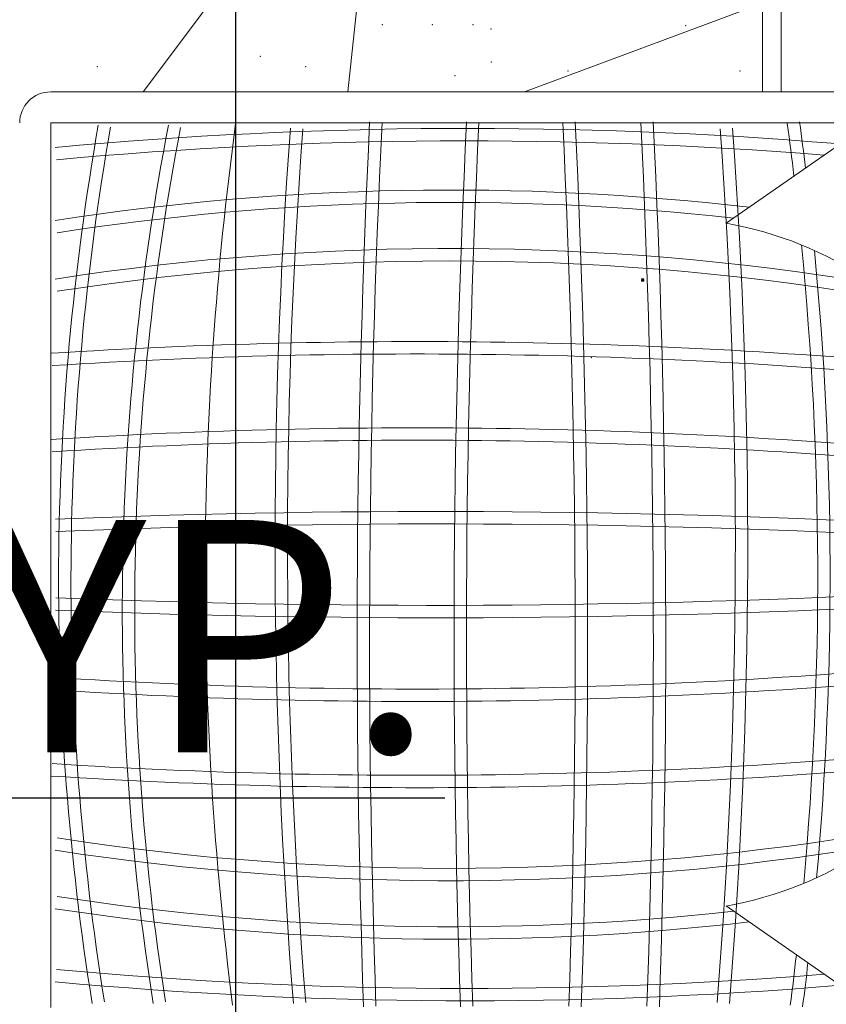
# Model space of a CAD drawing. Units: inches. Extents: x 1763 to 2368, y 1500 to 2097.
# Tile 19 of 24: x 2109 to 2152, y 1882 to 1935. Entities that reach past the tile are written whole.
import ezdxf

# ---------------------------------------------------------------- set-up
doc = ezdxf.new("R2010")
doc.units = ezdxf.units.IN
for name, color, linetype, lineweight in [('A-ANNO-DIMS', 2, 'Continuous', 18), ('A-FURN', 8, 'Continuous', 18), ('A-WALL-PATT', 7, 'Continuous', 13)]:
    doc.layers.add(name, color=color, linetype=linetype, lineweight=lineweight)
doc.styles.get("Standard").update_dxf_attribs({"font": 'arial.ttf'})
doc.dimstyles.new('ISO-25', dxfattribs={"dimtxt": 12.5, "dimasz": 2.5, "dimexe": 1.25, "dimexo": 0.625, "dimtad": 1, "dimdec": 0, "dimlunit": 4, "dimtxsty": 'Standard', "dimblk": 'ARCHTICK', "dimcen": 2.5, "dimclrd": 3, "dimclrt": 4, "dimadec": 0, "dimazin": 0, "dimtfac": 1, "dimtdec": 0, "dimtmove": 0, "dimatfit": 3, "dimfxl": 1, "dimarcsym": 0})

# ---------------------------------------------------------------- blocks, each defined once
blk = doc.blocks.new('A$C4CB008C5')
for p, q in [((0, 3), (0.6, 3)), ((0, 2.6), (0, 3)), ((0.6, 2.6), (0, 2.6)), ((0.1, 2.8), (0.5, 2.8)), ((0.1, 1.5), (0.6, 1.5)), ((0.1, 1.5), (0.1, 1.5)), ((0.1, 1.5), (0.1, 1.5)), ((0.1, 1.5), (0.1, 1.5)), ((0.1, 1.4), (0.1, 1.5)), ((0.1, 1.4), (0.1, 1.5)), ((0.1, 1.5), (0.1, 1.5)), ((0.1, 1.5), (0.1, 1.5)), ((0.1, 1.5), (0.1, 1.5)), ((0.1, 1.5), (0.1, 1.5)), ((0.1, 0), (0.1, 1.5)), ((0.1, 1.4), (0.1, 1.4)), ((0.1, 1.4), (0.1, 1.4)), ((0.1, 1.4), (0.1, 1.4)), ((0.1, 1.3), (0.1, 1.4)), ((0.1, 1.3), (0.1, 1.4)), ((0.1, 1.3), (0.1, 1.4)), ((0.1, 1.3), (0.1, 1.3)), ((0.1, 1.3), (0.1, 1.4)), ((0.1, 1.4), (0.1, 1.4)), ((0.1, 1.4), (0.1, 1.4)), ((0.1, 1.4), (0.1, 1.4)), ((0.1, 1.4), (0.1, 1.4)), ((0.1, 1.3), (0.1, 1.3)), ((0.1, 1.3), (0.1, 1.3)), ((0.1, 1.3), (0.1, 1.3)), ((0.1, 1.2), (0.1, 1.3)), ((0.1, 1.2), (0.1, 1.3)), ((0.1, 1.2), (0.1, 1.3)), ((0.1, 1.2), (0.1, 1.3)), ((0.1, 1.2), (0.1, 1.3)), ((0.1, 1.3), (0.1, 1.3)), ((0.1, 1.3), (0.1, 1.3)), ((0.1, 1.3), (0.1, 1.3)), ((0.1, 1.2), (0.1, 1.2)), ((0.1, 1.2), (0.1, 1.2)), ((0.1, 1.2), (0.1, 1.2)), ((0.1, 1.1), (0.1, 1.2)), ((0.1, 1.1), (0.1, 1.2)), ((0.1, 1.1), (0.1, 1.2)), ((0.1, 1.2), (0.1, 1.2)), ((0.1, 1.2), (0.1, 1.2)), ((0.1, 1.2), (0.1, 1.2)), ((0.1, 1.2), (0.1, 1.2)), ((0.1, 1.1), (0.1, 1.1)), ((0.1, 1.1), (0.1, 1.1)), ((0.1, 1.1), (0.1, 1.1)), ((0.1, 1), (0.1, 1.1)), ((0.1, 1), (0.1, 1.1)), ((0.1, 1), (0.1, 1)), ((0.1, 1), (0.1, 1.1)), ((0.1, 1.1), (0.1, 1.1)), ((0.1, 1.1), (0.1, 1.1)), ((0.1, 1.1), (0.1, 1.1)), ((0.1, 1), (0.1, 1)), ((0.1, 1), (0.1, 1)), ((0.1, 1), (0.1, 1)), ((0.1, 0.9), (0.1, 1)), ((0.1, 0.9), (0.1, 1)), ((0.1, 0.9), (0.1, 1)), ((0.1, 0.9), (0.1, 1)), ((0.1, 0.9), (0.1, 1)), ((0.1, 0.9), (0.1, 1)), ((0.1, 1), (0.1, 1)), ((0.1, 1), (0.1, 1)), ((0.1, 1), (0.1, 1)), ((0.1, 0.9), (0.1, 0.9)), ((0.1, 0.9), (0.1, 0.9)), ((0.1, 0.9), (0.1, 0.9)), ((0.1, 0.8), (0.1, 0.9)), ((0.1, 0.8), (0.1, 0.9)), ((0.1, 0.8), (0.1, 0.9)), ((0.1, 0.8), (0.1, 0.9)), ((0.1, 0.9), (0.1, 0.9)), ((0.1, 0.9), (0.1, 0.9)), ((0.1, 0.9), (0.1, 0.9)), ((0.1, 0.9), (0.1, 0.9)), ((0.1, 0.8), (0.1, 0.8)), ((0.1, 0.8), (0.1, 0.8)), ((0.1, 0.7), (0.1, 0.8)), ((0.1, 0.7), (0.1, 0.8)), ((0.1, 0.7), (0.1, 0.8)), ((0.1, 0.8), (0.1, 0.8)), ((0.1, 0.8), (0.1, 0.8)), ((0.1, 0.8), (0.1, 0.8)), ((0.1, 0.8), (0.1, 0.8)), ((0.1, 0.7), (0.1, 0.7)), ((0.1, 0.7), (0.1, 0.7)), ((0.1, 0.7), (0.1, 0.7)), ((0.1, 0.6), (0.1, 0.7)), ((0.1, 0.6), (0.1, 0.7)), ((0.1, 0.6), (0.1, 0.7)), ((0.1, 0.6), (0.1, 0.7)), ((0.1, 0.6), (0.1, 0.7)), ((0.1, 0.7), (0.1, 0.7)), ((0.1, 0.7), (0.1, 0.7)), ((0.1, 0.7), (0.1, 0.7)), ((0.1, 0.6), (0.1, 0.6)), ((0.1, 0.6), (0.1, 0.6)), ((0.1, 0.6), (0.1, 0.6)), ((0.1, 0.5), (0.1, 0.6)), ((0.1, 0.5), (0.1, 0.6)), ((0.1, 0.5), (0.1, 0.6)), ((0.1, 0.5), (0.1, 0.6)), ((0.1, 0.5), (0.1, 0.6)), ((0.1, 0.6), (0.1, 0.6)), ((0.1, 0.6), (0.1, 0.6)), ((0.1, 0.6), (0.1, 0.6)), ((0.1, 0.6), (0.1, 0.6)), ((0.1, 0.5), (0.1, 0.5)), ((0.1, 0.5), (0.1, 0.5)), ((0.1, 0.4), (0.1, 0.5)), ((0.1, 0.4), (0.1, 0.5)), ((0.1, 0.5), (0.1, 0.5)), ((0.1, 0.5), (0.1, 0.5)), ((0.1, 0.5), (0.1, 0.5)), ((0.1, 0.5), (0.1, 0.5)), ((0.1, 0.4), (0.1, 0.4)), ((0.1, 0.4), (0.1, 0.4)), ((0.1, 0.4), (0.1, 0.4)), ((0.1, 0.4), (0.1, 0.4)), ((0.1, 0.3), (0.1, 0.4)), ((0.1, 0.3), (0.1, 0.4)), ((0.1, 0.3), (0.1, 0.4)), ((0.1, 0.3), (0.1, 0.4)), ((0.1, 0.4), (0.1, 0.4)), ((0.1, 0.4), (0.1, 0.4)), ((0.1, 0.4), (0.1, 0.4)), ((0.1, 0.3), (0.1, 0.3)), ((0.1, 0.3), (0.1, 0.3)), ((0.1, 0.3), (0.1, 0.3)), ((0.1, 0.2), (0.1, 0.3)), ((0.1, 0.2), (0.1, 0.3)), ((0.1, 0.2), (0.1, 0.3)), ((0.1, 0.2), (0.1, 0.3)), ((0.1, 0.2), (0.1, 0.3)), ((0.1, 0.2), (0.1, 0.3)), ((0.1, 0.3), (0.1, 0.3)), ((0.1, 0.3), (0.1, 0.3)), ((0.1, 0.3), (0.1, 0.3)), ((0.1, 0.3), (0.1, 0.3)), ((0.1, 0.2), (0.1, 0.2)), ((0.1, 0.2), (0.1, 0.2)), ((0.1, 0.1), (0.1, 0.2)), ((0.1, 0.1), (0.1, 0.2)), ((0.1, 0.1), (0.1, 0.2)), ((0.1, 0.2), (0.1, 0.2)), ((0.1, 0.2), (0.1, 0.2)), ((0.1, 0.2), (0.1, 0.2)), ((0.1, 0.2), (0.1, 0.2)), ((0.1, 0.1), (0.1, 0.1)), ((0.1, 0.1), (0.1, 0.1)), ((0.1, 0.1), (0.1, 0.1)), ((0.1, 0), (0.1, 0.1)), ((0.1, 0), (0.1, 0.1)), ((0.1, 0.1), (0.1, 0.1)), ((0.1, 0), (0.1, 0.1)), ((0.1, 0.1), (0.1, 0.1)), ((0.1, 0.1), (0.1, 0.1)), ((0.1, 0.1), (0.1, 0.1)), ((0.1, 0), (0.1, 0)), ((0.1, 0), (0.1, 0)), ((0.1, 0), (0.1, 0)), ((0.1, 0), (0.1, 0)), ((0.1, 0), (0.1, 0)), ((0.1, 0), (0.1, 0)), ((0.1, 0), (0.1, 0)), ((0.3, 2.6), (0.3, 3)), ((0.3, 1.1), (0.5, 1.3)), ((0.7, 0.9), (0.3, 1.3)), ((0.3, 0.1), (0.3, 1.3)), ((0.3, 1.3), (0.6, 1.3)), ((0.3, 0.8), (0.6, 1.2)), ((0.6, 0.7), (0.3, 1)), ((0.3, 0.5), (0.6, 0.9)), ((0.9, 0.1), (0.3, 0.7)), ((0.3, 0.3), (0.6, 0.6)), ((0.6, 0.1), (0.3, 0.5)), ((0.3, 0.1), (0.3, 0.2)), ((3, 0.1), (0.3, 0.1)), ((0.6, 1.2), (0.5, 1.3)), ((0.5, 0.1), (0.8, 0.5)), ((0.6, 3), (2.6, 3)), ((0.6, 1.1), (0.6, 3)), ((0.6, 3), (2.6, 3)), ((0.6, 3), (0.6, 2.6)), ((0.6, 2.1), (1.9, 2.7)), ((0.6, 0.9), (0.6, 0.5)), ((2.5, 1), (0.7, 1)), ((0.7, 0.9), (0.8, 1)), ((0.7, 0.9), (2.6, 0.9)), ((0.7, 0.5), (2.6, 0.5)), ((0.7, 0.1), (1.1, 0.5)), ((0.8, 2.9), (1.6, 2.9)), ((0.8, 2.9), (2.5, 2.9)), ((0.8, 2.5), (0.8, 2.9)), ((0.8, 2.5), (0.8, 2.9)), ((0.8, 2.9), (0.8, 2.9)), ((1.6, 2.5), (0.8, 2.5)), ((0.8, 2.5), (0.8, 2.5)), ((1.5, 2.5), (0.8, 2.5)), ((1.2, 0.1), (0.8, 0.5)), ((0.9, 1.9), (1.9, 2.7)), ((0.9, 1.9), (0.9, 1.9)), ((1, 0.9), (0.9, 1)), ((1, 0.9), (1.1, 1)), ((1, 0.1), (1.4, 0.5)), ((1.2, 0.9), (1.1, 1)), ((1.4, 0.1), (1.1, 0.5)), ((1.2, 0.9), (1.3, 1)), ((1.3, 0.1), (1.6, 0.5)), ((1.5, 0.9), (1.4, 1)), ((1.7, 0.1), (1.4, 0.5)), ((1.5, 0.9), (1.6, 1)), ((1.6, 2.9), (1.6, 2.6)), ((1.6, 2.9), (1.7, 2.9)), ((1.6, 0.1), (1.9, 0.5)), ((1.7, 2.9), (1.7, 2.6)), ((1.7, 2.9), (1.7, 2.6)), ((1.7, 2.9), (2.5, 2.9)), ((1.7, 2.9), (1.7, 2.9)), ((1.8, 0.9), (1.7, 1)), ((2, 0.1), (1.7, 0.5)), ((1.8, 0.9), (1.9, 1)), ((1.9, 2.7), (2.6, 2.5)), ((1.9, 2.7), (2.5, 2.4)), ((1.9, 0.1), (2.2, 0.5)), ((2.1, 0.9), (2, 1)), ((2.3, 0.1), (2, 0.5)), ((2.1, 0.9), (2.2, 1)), ((2.2, 0.1), (2.5, 0.5)), ((2.4, 0.9), (2.3, 1)), ((2.6, 0.1), (2.3, 0.5)), ((2.4, 0.9), (2.5, 1)), ((2.4, 0.1), (3, 0.7)), ((2.5, 2.9), (2.5, 2.5)), ((2.5, 2.9), (2.5, 2.6)), ((2.5, 2.9), (2.5, 2.9)), ((2.9, 0.1), (2.5, 0.5)), ((2.6, 3), (2.6, 1.1)), ((2.6, 1.5), (3.2, 1.5)), ((2.6, 1.2), (2.8, 1.3)), ((2.6, 0.9), (3, 1.3)), ((2.6, 1.3), (3, 1.3)), ((3, 0.9), (2.6, 1.2)), ((2.6, 0.6), (3, 1)), ((3, 0.6), (2.6, 1)), ((2.6, 0.9), (2.6, 0.5)), ((3, 0.3), (2.6, 0.7)), ((3.3, 3), (2.7, 3)), ((2.7, 3), (2.7, 2.6)), ((2.7, 2.6), (3.3, 2.6)), ((2.7, 0.1), (3, 0.4)), ((3.2, 2.8), (2.8, 2.8)), ((3, 1.2), (2.8, 1.3)), ((3, 2.6), (3, 3)), ((3, 1.3), (3, 0.1)), ((3.2, 1.5), (3.1, 1.5)), ((3.1, 1.5), (3.1, 1.5)), ((3.1, 1.5), (3.2, 1.5)), ((3.1, 1.5), (3.2, 1.5)), ((3.1, 1.5), (3.1, 0)), ((3.2, 1.3), (3.1, 1.4)), ((3.2, 1.3), (3.1, 1.4)), ((3.2, 1.3), (3.1, 1.4)), ((3.2, 1.4), (3.1, 1.4)), ((3.2, 1.4), (3.1, 1.4)), ((3.1, 1.4), (3.1, 1.4)), ((3.1, 1.4), (3.2, 1.4)), ((3.1, 1.4), (3.2, 1.4)), ((3.1, 1.4), (3.2, 1.4)), ((3.1, 1.3), (3.2, 1.4)), ((3.1, 1.3), (3.2, 1.3)), ((3.2, 1.2), (3.1, 1.3)), ((3.2, 1.2), (3.1, 1.3)), ((3.2, 1.3), (3.1, 1.3)), ((3.1, 1.3), (3.1, 1.3)), ((3.1, 1.2), (3.2, 1.3)), ((3.1, 1.2), (3.2, 1.3)), ((3.1, 1.2), (3.2, 1.3)), ((3.2, 1.1), (3.1, 1.2)), ((3.2, 1.2), (3.1, 1.2)), ((3.2, 1.2), (3.1, 1.2)), ((3.1, 1.2), (3.2, 1.2)), ((3.1, 1.2), (3.2, 1.2)), ((3.1, 1.2), (3.1, 1.2)), ((3.1, 1.1), (3.2, 1.2)), ((3.2, 1), (3.1, 1.1)), ((3.2, 1), (3.1, 1.1)), ((3.2, 1.1), (3.1, 1.1)), ((3.2, 1.1), (3.1, 1.1)), ((3.1, 1.1), (3.2, 1.1)), ((3.1, 1.1), (3.2, 1.1)), ((3.1, 1.1), (3.2, 1.1)), ((3.1, 1), (3.2, 1.1)), ((3.2, 0.9), (3.1, 1)), ((3.2, 0.9), (3.1, 1)), ((3.2, 0.9), (3.1, 1)), ((3.2, 1), (3.1, 1)), ((3.1, 1), (3.1, 1)), ((3.1, 1), (3.2, 1)), ((3.1, 0.9), (3.2, 1)), ((3.1, 0.9), (3.2, 1)), ((3.1, 0.9), (3.2, 1)), ((3.2, 0.8), (3.1, 0.9)), ((3.2, 0.8), (3.1, 0.9)), ((3.2, 0.9), (3.1, 0.9)), ((3.1, 0.9), (3.2, 0.9)), ((3.1, 0.9), (3.1, 0.9)), ((3.1, 0.8), (3.2, 0.9)), ((3.1, 0.8), (3.2, 0.9)), ((3.2, 0.7), (3.1, 0.8)), ((3.2, 0.8), (3.1, 0.8)), ((3.2, 0.8), (3.1, 0.8)), ((3.1, 0.8), (3.2, 0.8)), ((3.1, 0.8), (3.2, 0.8)), ((3.1, 0.8), (3.2, 0.8)), ((3.2, 0.6), (3.1, 0.7)), ((3.2, 0.6), (3.1, 0.7)), ((3.2, 0.6), (3.1, 0.7)), ((3.2, 0.7), (3.1, 0.7)), ((3.2, 0.7), (3.1, 0.7)), ((3.1, 0.7), (3.1, 0.7)), ((3.1, 0.7), (3.2, 0.7)), ((3.1, 0.7), (3.2, 0.7)), ((3.1, 0.6), (3.2, 0.7)), ((3.1, 0.6), (3.2, 0.7)), ((3.2, 0.5), (3.1, 0.6)), ((3.2, 0.5), (3.1, 0.6)), ((3.2, 0.6), (3.1, 0.6)), ((3.1, 0.6), (3.2, 0.6)), ((3.1, 0.6), (3.1, 0.6)), ((3.1, 0.5), (3.2, 0.6)), ((3.1, 0.5), (3.2, 0.6)), ((3.1, 0.5), (3.2, 0.6)), ((3.2, 0.5), (3.1, 0.5)), ((3.2, 0.5), (3.1, 0.5)), ((3.1, 0.5), (3.2, 0.5)), ((3.1, 0.5), (3.2, 0.5)), ((3.1, 0.5), (3.1, 0.5)), ((3.2, 0.3), (3.1, 0.4)), ((3.2, 0.3), (3.1, 0.4)), ((3.2, 0.4), (3.1, 0.4)), ((3.2, 0.4), (3.1, 0.4)), ((3.2, 0.4), (3.1, 0.4)), ((3.1, 0.4), (3.2, 0.4)), ((3.1, 0.4), (3.2, 0.4)), ((3.1, 0.4), (3.2, 0.4)), ((3.1, 0.3), (3.2, 0.4)), ((3.1, 0.3), (3.2, 0.4)), ((3.2, 0.2), (3.1, 0.3)), ((3.2, 0.2), (3.1, 0.3)), ((3.2, 0.2), (3.1, 0.3)), ((3.2, 0.3), (3.1, 0.3)), ((3.1, 0.3), (3.1, 0.3)), ((3.1, 0.3), (3.2, 0.3)), ((3.1, 0.2), (3.2, 0.3)), ((3.1, 0.2), (3.2, 0.3)), ((3.1, 0.2), (3.2, 0.3)), ((3.2, 0.1), (3.1, 0.2)), ((3.2, 0.2), (3.1, 0.2)), ((3.1, 0.2), (3.2, 0.2)), ((3.1, 0.2), (3.1, 0.2)), ((3.1, 0.1), (3.2, 0.2)), ((3.2, 0), (3.1, 0.1)), ((3.2, 0.1), (3.1, 0.1)), ((3.2, 0.1), (3.1, 0.1)), ((3.2, 0.1), (3.1, 0.1)), ((3.1, 0.1), (3.2, 0.1)), ((3.1, 0.1), (3.2, 0.1)), ((3.1, 0.1), (3.2, 0.1)), ((3.1, 0), (3.2, 0.1)), ((3.1, 0), (3.1, 0)), ((3.2, 0), (3.1, 0)), ((3.1, 0), (3.1, 0)), ((3.2, 1.4), (3.2, 1.5)), ((3.2, 1.5), (3.2, 1.5)), ((3.2, 1.5), (3.2, 1.5)), ((3.2, 1.5), (3.2, 1.5)), ((3.2, 1.4), (3.2, 1.5)), ((3.2, 1.4), (3.2, 1.4)), ((3.2, 1.3), (3.2, 1.3)), ((3.2, 1.3), (3.2, 1.3)), ((3.2, 1.3), (3.2, 1.3)), ((3.2, 1.3), (3.2, 1.3)), ((3.2, 1.2), (3.2, 1.2)), ((3.2, 1.2), (3.2, 1.2)), ((3.2, 1.1), (3.2, 1.2)), ((3.2, 1.1), (3.2, 1.1)), ((3.2, 1), (3.2, 1)), ((3.2, 1), (3.2, 1)), ((3.2, 1), (3.2, 1)), ((3.2, 1), (3.2, 1)), ((3.2, 0.9), (3.2, 0.9)), ((3.2, 0.9), (3.2, 0.9)), ((3.2, 0.9), (3.2, 0.9)), ((3.2, 0.9), (3.2, 0.9)), ((3.2, 0.7), (3.2, 0.8)), ((3.2, 0.8), (3.2, 0.8)), ((3.2, 0.7), (3.2, 0.8)), ((3.2, 0.7), (3.2, 0.7)), ((3.2, 0.6), (3.2, 0.6)), ((3.2, 0.6), (3.2, 0.6)), ((3.2, 0.6), (3.2, 0.6)), ((3.2, 0.6), (3.2, 0.6)), ((3.2, 0.4), (3.2, 0.5)), ((3.2, 0.5), (3.2, 0.5)), ((3.2, 0.4), (3.2, 0.5)), ((3.2, 0.4), (3.2, 0.4)), ((3.2, 0.3), (3.2, 0.3)), ((3.2, 0.3), (3.2, 0.3)), ((3.2, 0.3), (3.2, 0.3)), ((3.2, 0.3), (3.2, 0.3)), ((3.2, 0.1), (3.2, 0.2)), ((3.2, 0.2), (3.2, 0.2)), ((3.2, 0.2), (3.2, 0.2)), ((3.2, 0.2), (3.2, 0.2)), ((3.2, 0), (3.2, 0.1)), ((3.2, 0.1), (3.2, 0.1)), ((3.2, 0), (3.2, 0)), ((3.2, 0), (3.2, 0)), ((3.2, 0), (3.2, 0)), ((3.2, 0), (3.2, 0)), ((3.3, 2.6), (3.3, 3)), ((0.1, 0), (3.2, 0))]:
    blk.add_line(p, q)
for centre, radius in [((0.3, 2.8), 0.15), ((0.3, 2.8), 0.05), ((3, 2.8), 0.15), ((3, 2.8), 0.05)]:
    blk.add_circle(centre, radius)
for centre, radius, start, end in [((0.7, 1.9), 0.207, 354.6422, 106.9775), ((0.7, 1.1), 0.1, 180, 270), ((0.7, 0.9), 0.05, 90, 180), ((0.7, 0.5), 0.05, 180, 270), ((1.9, 2.6), 0.1, 71.7215, 119.0799), ((2.6, 2.3), 0.198, 84.1725, 146.9889), ((2.5, 1.1), 0.1, 270, 0), ((2.6, 0.9), 0.05, 0, 90), ((2.6, 0.5), 0.05, 270, 0)]:
    blk.add_arc(centre, radius, start, end)
blk = doc.blocks.new('A$C77DF40FE')
for p, q in [((0.5339, 0.6344), (0.5339, 2.6214)), ((0.5839, 0.6344), (0.5839, 2.6214)), ((0.6051, 1.925), (0.7457, 1.7234)), ((1.9869, 1.925), (1.8463, 1.7234)), ((0.5339, 1.8116), (0.3112, 1.8116)), ((0.5339, 1.7816), (0.3112, 1.7816)), ((0.3909, 1.7821), (0.5339, 1.398)), ((0.5339, 1.1132), (0.2152, 1.1479)), ((0.5339, 0.7837), (0.2152, 1.0221)), ((2.0097, 0.6344), (0.5839, 0.6344))]:
    blk.add_line(p, q)
for centre, radius, start, end in [((1.3217, 1.6229), 0.5847, 121.6676, 170.1065), ((10.1174, 1.2237), 9.161, 174.43278, 183.67204), ((10.2564, 1.2237), 9.181, 174.43278, 183.67204), ((10.2564, 1.2237), 9.161, 174.43278, 183.67204), ((16.3019, 1.253), 15.0916, 176.72768, 182.32074), ((16.3019, 1.253), 15.0716, 176.72768, 182.32074), ((-13.7099, 1.253), 15.0716, 357.67926, 3.27232), ((-13.7099, 1.253), 15.0916, 357.67926, 3.27232), ((-7.6644, 1.2237), 9.161, 356.32796, 5.56722), ((-7.6644, 1.2237), 9.181, 356.32796, 5.56722), ((1.2703, 1.6229), 0.5847, 9.8935, 58.3324), ((10.1174, 1.2237), 9.181, 174.54912, 183.67204), ((-7.5254, 1.2237), 9.161, 356.32796, 5.55658), ((-7.5254, 1.2237), 9.181, 356.32796, 5.45088), ((4.947, 1.2796), 4.1406, 170.0939, 188.8179), ((-2.355, 1.2796), 4.1406, 351.1821, 9.9061), ((4.947, 1.2796), 4.1606, 170.6272, 188.8179), ((-2.355, 1.2796), 4.1606, 351.1821, 9.3728), ((7.8077, 1.3061), 7.2149, 175.27403, 185.28261), ((1.3142, -3.5764), 5.4671, 84.8953, 95.5052), ((-5.2157, 1.3061), 7.2149, 354.71739, 4.72597), ((7.8077, 1.3061), 7.1949, 175.41729, 185.28261), ((-5.2157, 1.3061), 7.1949, 354.71739, 4.58271), ((1.3142, -3.5764), 5.4471, 84.7792, 95.6214), ((1.3142, -3.5764), 5.4671, 96.9078, 97.6924), ((1.3142, -3.5764), 5.4671, 82.7025, 83.4474), ((1.3142, -3.5764), 5.4471, 96.796, 97.6924), ((1.3142, -3.5764), 5.4471, 82.7025, 83.5609), ((1.2659, -7.4764), 9.2344, 85.41732, 94.18368), ((4.8527, 1.2796), 4.1606, 173.3677, 188.8179), ((-2.2608, 1.2796), 4.1606, 351.1821, 6.6323), ((1.2659, -7.4764), 9.2144, 85.41732, 94.18368), ((4.8527, 1.2796), 4.1406, 173.6812, 188.8179), ((-2.2608, 1.2796), 4.1406, 351.1821, 6.3188), ((1.4138, -15.5462), 17.172, 88.01473, 92.775), ((1.4138, -15.5462), 17.152, 88.01473, 92.775), ((1.4138, -15.6721), 17.172, 88.01473, 92.775), ((1.4138, -15.6721), 17.152, 88.01473, 92.775), ((1.4138, 18.4566), 17.152, 267.225, 271.98527), ((1.4138, 18.4566), 17.172, 267.225, 271.98527), ((1.4138, 18.3004), 17.152, 267.225, 271.98527), ((1.4138, 18.3004), 17.172, 267.225, 271.98527), ((1.2659, 10.2305), 9.2144, 265.81632, 274.58268), ((1.2659, 10.2305), 9.2344, 265.81632, 274.58268), ((1.3142, 6.3306), 5.4471, 262.3076, 277.2975), ((1.3657, 4.8586), 4.0888, 259.0794, 278.9327), ((1.3657, 4.8586), 4.1088, 259.0794, 278.9327), ((1.3248, 4.9264), 4.2593, 260.0761, 279.1287), ((1.3248, 4.9264), 4.2793, 260.0761, 279.1287), ((0.5839, 0.6344), 0.05, 180, 270)]:
    blk.add_arc(centre, radius, start, end)
for p in [(0.5004, 1.7457), (0.4274, 1.6581), (0.9622, 1.5058), (0.5004, 1.4684), (0.4326, 1.3443), (0.4858, 1.3444), (0.4253, 1.3151), (0.5077, 1.286), (0.4253, 1.2495), (0.4253, 1.1692), (0.4931, 1.0452), (0.4765, 0.9722), (0.4931, 0.7096)]:
    blk.add_point(p)
blk = doc.blocks.new('_ArchTick')
at = {"color": 0, "linetype": 'ByBlock', "const_width": 0.15}
blk.add_lwpolyline([(-0.5, -0.5), (0.5, 0.5)], dxfattribs=at)
blk = doc.blocks.new('*D23')
at = {"layer": 'A-ANNO-DIMS', "color": 0, "lineweight": -2, "transparency": 16777216}
for p, q in [((2089.477, 1949.977), (2089.477, 1963.985)), ((2178.698, 1949.977), (2178.698, 1963.985))]:
    blk.add_line(p, q, dxfattribs=at)
at = {"layer": 'A-ANNO-DIMS', "color": 3, "lineweight": -2, "transparency": 16777216}
for p, q in [((2089.477, 1962.735), (2178.698, 1962.735)), ((2178.698, 1962.735), (2367.732, 1962.735))]:
    blk.add_line(p, q, dxfattribs=at)
at = {"layer": 'Defpoints', "color": 0, "transparency": 16777216}
for p in [(2178.698, 1962.735), (2089.477, 1949.352), (2178.698, 1949.352)]:
    blk.add_point(p, dxfattribs=at)
at = {"layer": 'A-ANNO-DIMS', "color": 3, "lineweight": -2, "transparency": 16777216, "xscale": 2.5, "yscale": 2.5, "zscale": 2.5, "rotation": 180}
blk.add_blockref('_ArchTick', (2089.477, 1962.735), dxfattribs=at)
at = {"layer": 'A-ANNO-DIMS', "color": 3, "lineweight": -2, "transparency": 16777216, "xscale": 2.5, "yscale": 2.5, "zscale": 2.5}
blk.add_blockref('_ArchTick', (2178.698, 1962.735), dxfattribs=at)
at = {"layer": 'A-ANNO-DIMS', "color": 4, "transparency": 16777216, "insert": (2274.465, 1969.828), "char_height": 12.5, "attachment_point": 5}
blk.add_mtext('BED GROUP 7\'-5" TYP.', dxfattribs=at)
blk = doc.blocks.new('*D34')
at = {"layer": 'A-ANNO-DIMS', "color": 0, "lineweight": -2, "transparency": 16777216}
for p, q in [((2001.644, 1895.481), (2001.644, 1892.281)), ((2013.092, 1895.481), (2013.092, 1892.281))]:
    blk.add_line(p, q, dxfattribs=at)
at = {"layer": 'A-ANNO-DIMS', "color": 3, "lineweight": -2, "transparency": 16777216}
for p, q in [((2001.644, 1893.531), (2013.092, 1893.531)), ((2013.092, 1893.531), (2131.874, 1893.531))]:
    blk.add_line(p, q, dxfattribs=at)
at = {"layer": 'Defpoints', "color": 0, "transparency": 16777216}
for p in [(2001.644, 1896.106), (2013.092, 1896.106), (2013.092, 1893.531)]:
    blk.add_point(p, dxfattribs=at)
at = {"layer": 'A-ANNO-DIMS', "color": 3, "lineweight": -2, "transparency": 16777216, "xscale": 2.5, "yscale": 2.5, "zscale": 2.5, "rotation": 180}
blk.add_blockref('_ArchTick', (2001.644, 1893.531), dxfattribs=at)
at = {"layer": 'A-ANNO-DIMS', "color": 3, "lineweight": -2, "transparency": 16777216, "xscale": 2.5, "yscale": 2.5, "zscale": 2.5}
blk.add_blockref('_ArchTick', (2013.092, 1893.531), dxfattribs=at)
at = {"layer": 'A-ANNO-DIMS', "color": 4, "transparency": 16777216, "insert": (2073.733, 1900.619), "char_height": 12.5, "attachment_point": 5}
blk.add_mtext('0\'-11 1/2" TYP.', dxfattribs=at)
blk = doc.blocks.new('*D62')
at = {"layer": 'A-ANNO-DIMS', "color": 0, "lineweight": -2, "transparency": 16777216}
for p, q in [((2083.092, 1980.648), (2083.092, 1509.906)), ((2120.612, 1980.648), (2120.612, 1509.906))]:
    blk.add_line(p, q, dxfattribs=at)
at = {"layer": 'A-ANNO-DIMS', "color": 3, "lineweight": -2, "transparency": 16777216}
for p, q in [((2083.092, 1511.156), (2120.612, 1511.156)), ((2120.612, 1511.156), (2186.709, 1511.156))]:
    blk.add_line(p, q, dxfattribs=at)
at = {"layer": 'Defpoints', "color": 0, "transparency": 16777216}
for p in [(2083.092, 1981.273), (2120.612, 1981.273), (2120.612, 1511.156)]:
    blk.add_point(p, dxfattribs=at)
at = {"layer": 'A-ANNO-DIMS', "color": 3, "lineweight": -2, "transparency": 16777216, "xscale": 2.5, "yscale": 2.5, "zscale": 2.5, "rotation": 180}
blk.add_blockref('_ArchTick', (2083.092, 1511.156), dxfattribs=at)
at = {"layer": 'A-ANNO-DIMS', "color": 3, "lineweight": -2, "transparency": 16777216, "xscale": 2.5, "yscale": 2.5, "zscale": 2.5}
blk.add_blockref('_ArchTick', (2120.612, 1511.156), dxfattribs=at)
at = {"layer": 'A-ANNO-DIMS', "color": 4, "transparency": 16777216, "insert": (2154.91, 1518.249), "char_height": 12.5, "attachment_point": 5}
blk.add_mtext('3\'-1 1/2"', dxfattribs=at)
blk = doc.blocks.new('*D72')
at = {"layer": 'A-ANNO-DIMS', "color": 0, "lineweight": -2, "transparency": 16777216}
for p, q in [((2018.092, 1885.898), (2018.092, 2072.023)), ((2049.737, 1885.898), (2049.737, 2072.023))]:
    blk.add_line(p, q, dxfattribs=at)
at = {"layer": 'A-ANNO-DIMS', "color": 3, "lineweight": -2, "transparency": 16777216}
for p, q in [((2018.092, 2070.773), (2049.737, 2070.773)), ((2049.737, 2070.773), (2116.055, 2070.773))]:
    blk.add_line(p, q, dxfattribs=at)
at = {"layer": 'Defpoints', "color": 0, "transparency": 16777216}
for p in [(2049.737, 2070.773), (2018.092, 1885.273), (2049.737, 1885.273)]:
    blk.add_point(p, dxfattribs=at)
at = {"layer": 'A-ANNO-DIMS', "color": 3, "lineweight": -2, "transparency": 16777216, "xscale": 2.5, "yscale": 2.5, "zscale": 2.5, "rotation": 180}
blk.add_blockref('_ArchTick', (2018.092, 2070.773), dxfattribs=at)
at = {"layer": 'A-ANNO-DIMS', "color": 3, "lineweight": -2, "transparency": 16777216, "xscale": 2.5, "yscale": 2.5, "zscale": 2.5}
blk.add_blockref('_ArchTick', (2049.737, 2070.773), dxfattribs=at)
at = {"layer": 'A-ANNO-DIMS', "color": 4, "transparency": 16777216, "insert": (2084.146, 2077.861), "char_height": 12.5, "attachment_point": 5}
blk.add_mtext('2\'-7 1/2"', dxfattribs=at)
blk = doc.blocks.new('*D78')
at = {"layer": 'A-ANNO-DIMS', "color": 0, "lineweight": -2, "transparency": 16777216}
for p, q in [((1996.717, 1981.273), (2217.842, 1981.273)), ((1986.217, 1948.273), (2217.842, 1948.273))]:
    blk.add_line(p, q, dxfattribs=at)
at = {"layer": 'A-ANNO-DIMS', "color": 3, "lineweight": -2, "transparency": 16777216}
for p, q in [((2216.592, 1981.273), (2216.592, 1948.273)), ((2216.592, 1948.273), (2216.592, 1911.081))]:
    blk.add_line(p, q, dxfattribs=at)
at = {"layer": 'Defpoints', "color": 0, "transparency": 16777216}
for p in [(1996.092, 1981.273), (1985.592, 1948.273), (2216.592, 1948.273)]:
    blk.add_point(p, dxfattribs=at)
at = {"layer": 'A-ANNO-DIMS', "color": 3, "lineweight": -2, "transparency": 16777216, "xscale": 2.5, "yscale": 2.5, "zscale": 2.5}
for p, rotation in [((2216.592, 1981.273), 90), ((2216.592, 1948.273), 270)]:
    blk.add_blockref('_ArchTick', p, dxfattribs=dict(at, rotation=rotation))
at = {"layer": 'A-ANNO-DIMS', "color": 4, "transparency": 16777216, "insert": (2209.585, 1928.427), "char_height": 12.5, "attachment_point": 5, "rotation": 90}
blk.add_mtext('2\'-9"', dxfattribs=at)
blk = doc.blocks.new('*D95')
at = {"layer": 'A-ANNO-DIMS', "color": 0, "lineweight": -2, "transparency": 16777216}
for p, q in [((2125.159, 1998.768), (2217.842, 1998.768)), ((2121.237, 1986.273), (2217.842, 1986.273))]:
    blk.add_line(p, q, dxfattribs=at)
at = {"layer": 'A-ANNO-DIMS', "color": 3, "lineweight": -2, "transparency": 16777216}
for p, q in [((2216.592, 1998.768), (2216.592, 1986.273)), ((2216.592, 1986.273), (2216.592, 1921.344))]:
    blk.add_line(p, q, dxfattribs=at)
at = {"layer": 'Defpoints', "color": 0, "transparency": 16777216}
for p in [(2124.534, 1998.768), (2120.612, 1986.273), (2216.592, 1986.273)]:
    blk.add_point(p, dxfattribs=at)
at = {"layer": 'A-ANNO-DIMS', "color": 3, "lineweight": -2, "transparency": 16777216, "xscale": 2.5, "yscale": 2.5, "zscale": 2.5}
for p, rotation in [((2216.592, 1998.768), 90), ((2216.592, 1986.273), 270)]:
    blk.add_blockref('_ArchTick', p, dxfattribs=dict(at, rotation=rotation))
at = {"layer": 'A-ANNO-DIMS', "color": 4, "transparency": 16777216, "insert": (2209.504, 1952.559), "char_height": 12.5, "attachment_point": 5, "rotation": 90}
blk.add_mtext('1\'-0 1/2"', dxfattribs=at)

msp = doc.modelspace()

# ---------------------------------------------------------------- hatches: boundary and pattern name
at = {"layer": 'A-WALL-PATT'}
h = msp.add_hatch(color=256, dxfattribs=at)
h.dxf.hatch_style = 1
h.paths.add_polyline_path([(1838.092, 2034.273), (1838.092, 2043.273), (1829.092, 2043.273), (1829.092, 1953.387), (1838.092, 1953.387)])
h.paths.add_polyline_path([(1838.092, 1913.101), (1829.092, 1913.101), (1829.092, 1862.202), (1838.092, 1862.202)])
h.paths.add_polyline_path([(1838.092, 1825.59), (1829.092, 1825.59), (1829.092, 1738.643), (1838.092, 1738.643)])
h.paths.add_polyline_path([(1895.592, 1885.273), (1838.092, 1885.273), (1838.092, 1880.273), (1895.592, 1880.273)])
h.paths.add_polyline_path([(1857.389, 1784.273), (1838.092, 1784.273), (1838.092, 1779.273), (1857.389, 1779.273)])
h.paths.add_polyline_path([(1958.092, 1981.273), (1971.455, 1981.273), (1971.455, 1986.273), (1968.568, 1986.273), (1958.092, 1986.273), (1953.092, 1986.273), (1927.39, 1986.273), (1927.39, 1981.273), (1953.092, 1981.273), (1953.092, 1885.273), (1932.014, 1885.273), (1932.014, 1880.273), (1959.134, 1880.273), (1959.134, 1883.738), (1959.134, 1885.273), (1958.092, 1885.273)])
h.paths.add_polyline_path([(2018.092, 1981.273), (2031.019, 1981.273), (2031.019, 1986.273), (2018.092, 1986.273), (2013.092, 1986.273), (2001.233, 1986.273), (2001.233, 1981.273), (2013.092, 1981.273), (2013.092, 1885.273), (1982.182, 1885.273, -0.016629), (1982.233, 1883.738), (1982.233, 1880.273), (2049.686, 1880.273), (2049.686, 1883.738, -0.016629), (2049.737, 1885.273), (2018.092, 1885.273)])
h.paths.add_polyline_path([(2083.092, 1981.273), (2120.612, 1981.273), (2120.612, 1986.273), (2083.092, 1986.273), (2078.092, 1986.273), (2063.143, 1986.273), (2063.143, 1981.273), (2078.092, 1981.273), (2078.092, 1885.273), (2072.785, 1885.273), (2072.785, 1883.738), (2072.785, 1880.273), (2078.092, 1880.273), (2078.092, 1866.867), (2081.557, 1866.867, -0.016629), (2083.092, 1866.816)])
h.paths.add_polyline_path([(1871.675, 1635.273), (1838.092, 1635.273), (1838.092, 1626.273), (1871.675, 1626.273)], flags=17)
h.paths.add_polyline_path([(2100.577, 1688.273), (2060.092, 1688.273), (2060.092, 1679.273), (2100.577, 1679.273)], flags=17)
h.paths.add_polyline_path([(2180.092, 1688.273), (2148.744, 1688.273), (2148.744, 1679.273), (2180.092, 1679.273)], flags=17)
h.paths.add_polyline_path([(2189.092, 1746.219), (2180.092, 1746.219), (2180.092, 1743.417), (2180.123, 1743.417), (2180.123, 1726.723), (2180.092, 1572.273), (2034.907, 1572.273), (2034.907, 1565.601), (2034.907, 1563.273), (2189.092, 1563.273)])
h.paths.add_polyline_path([(2060.092, 1802.347, -0.016629), (2058.557, 1802.296), (2055.092, 1802.296), (2055.092, 1635.273), (2042.484, 1635.273), (2042.484, 1629.738), (2042.484, 1626.273), (2055.092, 1626.273), (2055.092, 1599.273), (2040.269, 1599.273), (2040.269, 1590.273), (2060.092, 1590.273)])
h.paths.add_polyline_path([(2019.385, 1629.738, -0.060569), (2020.058, 1635.273), (1995.092, 1635.273), (1990.092, 1635.273), (1927.075, 1635.273), (1927.075, 1626.273), (1990.092, 1626.273), (1990.092, 1590.273), (1995.092, 1590.273), (2005.195, 1590.273), (2005.195, 1599.273), (1995.092, 1599.273), (1995.092, 1626.273), (2019.385, 1626.273)])
edge = h.paths.add_edge_path()
edge.add_line((2180.092, 1837.273), (2167.198, 1837.273))
edge.add_spline(control_points=[(2167.198, 1837.273), (2167.191, 1837.271), (2167.183, 1837.271), (2167.176, 1837.273)], knot_values=[168.955493, 168.955493, 168.955493, 168.955493, 169.065871, 169.065871, 169.065871, 169.065871], degree=3, periodic=0)
edge.add_spline(control_points=[(2167.176, 1837.273), (2166.556, 1837.377), (2166.326, 1846.161), (2165.708, 1846.244)], knot_values=[159.864705, 159.864705, 159.864705, 159.864705, 168.955493, 168.955493, 168.955493, 168.955493], degree=3, periodic=0)
edge.add_line((2167.122, 1837.273), (2163.16, 1837.273))
edge.add_spline(control_points=[(2163.16, 1837.273), (2163.158, 1837.273), (2163.156, 1837.273), (2163.155, 1837.273)], knot_values=[150.537172, 150.537172, 150.537172, 150.537172, 150.553797, 150.553797, 150.553797, 150.553797], degree=3, periodic=0)
edge.add_spline(control_points=[(2163.155, 1837.273), (2162.29, 1837.289), (2161.594, 1846.232), (2160.878, 1846.244)], knot_values=[141.293426, 141.293426, 141.293426, 141.293426, 150.537172, 150.537172, 150.537172, 150.537172], degree=3, periodic=0)
edge.add_line((2163.075, 1837.273), (2158.7, 1837.273))
edge.add_spline(control_points=[(2158.7, 1837.273), (2158.698, 1837.273), (2158.697, 1837.273), (2158.696, 1837.273)], knot_values=[132.033544, 132.033544, 132.033544, 132.033544, 132.049151, 132.049151, 132.049151, 132.049151], degree=3, periodic=0)
edge.add_spline(control_points=[(2158.696, 1837.273), (2157.972, 1837.288), (2157.262, 1846.233), (2156.393, 1846.244)], knot_values=[122.786021, 122.786021, 122.786021, 122.786021, 132.033544, 132.033544, 132.033544, 132.033544], degree=3, periodic=0)
edge.add_line((2158.629, 1837.273), (2153.839, 1837.273))
edge.add_spline(control_points=[(2153.839, 1837.273), (2153.831, 1837.271), (2153.823, 1837.271), (2153.816, 1837.273)], knot_values=[113.451585, 113.451585, 113.451585, 113.451585, 113.562103, 113.562103, 113.562103, 113.562103], degree=3, periodic=0)
edge.add_spline(control_points=[(2153.816, 1837.273), (2153.17, 1837.378), (2152.878, 1846.191), (2152.404, 1846.244)], knot_values=[0, 0, 0, 0, 9.081854, 9.081854, 9.081854, 9.081854], degree=3, periodic=0)
edge.add_line((2153.76, 1837.273), (2150.391, 1837.273))
edge.add_spline(control_points=[(2150.391, 1837.273), (2150.381, 1837.272), (2150.371, 1837.272), (2150.361, 1837.273)], knot_values=[95.069382, 95.069382, 95.069382, 95.069382, 95.17519, 95.17519, 95.17519, 95.17519], degree=3, periodic=0)
edge.add_spline(control_points=[(2150.361, 1837.273), (2149.487, 1837.373), (2148.419, 1846.194), (2147.589, 1846.244)], knot_values=[85.824599, 85.824599, 85.824599, 85.824599, 95.069382, 95.069382, 95.069382, 95.069382], degree=3, periodic=0)
edge.add_line((2150.286, 1837.273), (2145.43, 1837.273))
edge.add_spline(control_points=[(2145.43, 1837.273), (2145.426, 1837.273), (2145.423, 1837.273), (2145.419, 1837.273)], knot_values=[76.505559, 76.505559, 76.505559, 76.505559, 76.547811, 76.547811, 76.547811, 76.547811], degree=3, periodic=0)
edge.add_spline(control_points=[(2145.419, 1837.273), (2144.684, 1837.313), (2143.804, 1846.194), (2142.948, 1846.244)], knot_values=[67.23945, 67.23945, 67.23945, 67.23945, 76.505559, 76.505559, 76.505559, 76.505559], degree=3, periodic=0)
edge.add_line((2145.353, 1837.273), (2134.57, 1837.273))
edge.add_spline(control_points=[(2134.57, 1837.273), (2134.567, 1837.272), (2134.563, 1837.272), (2134.56, 1837.273)], knot_values=[39.001463, 39.001463, 39.001463, 39.001463, 39.045107, 39.045107, 39.045107, 39.045107], degree=3, periodic=0)
edge.add_spline(control_points=[(2134.56, 1837.273), (2133.872, 1837.313), (2133.397, 1845.853), (2132.328, 1846.244)], knot_values=[29.79778, 29.79778, 29.79778, 29.79778, 39.001463, 39.001463, 39.001463, 39.001463], degree=3, periodic=0)
edge.add_line((2134.498, 1837.273), (2128.075, 1837.273))
edge.add_spline(control_points=[(2128.075, 1837.273), (2128.026, 1837.26), (2127.978, 1837.26), (2127.931, 1837.273)], knot_values=[19.482067, 19.482067, 19.482067, 19.482067, 19.869396, 19.869396, 19.869396, 19.869396], degree=3, periodic=0)
edge.add_spline(control_points=[(2125.013, 1846.244), (2126.165, 1844.663), (2126.821, 1837.57), (2127.931, 1837.273)], knot_values=[10.389805, 10.389805, 10.389805, 10.389805, 19.482067, 19.482067, 19.482067, 19.482067], degree=3, periodic=0)
edge.add_line((2127.931, 1837.273), (2083.092, 1837.273))
edge.add_line((2083.092, 1837.273), (2083.092, 1843.768))
edge.add_line((2083.092, 1843.768), (2081.557, 1843.768))
edge.add_line((2081.557, 1843.768), (2078.092, 1843.768))
edge.add_line((2078.092, 1843.768), (2078.092, 1837.273))
edge.add_line((2078.092, 1837.273), (2055.092, 1837.273))
edge.add_line((2055.092, 1837.273), (2055.092, 1825.395))
edge.add_line((2055.092, 1825.395), (2058.557, 1825.395))
edge.add_line((2058.557, 1825.395), (2060.092, 1825.395))
edge.add_line((2060.092, 1825.395), (2060.092, 1832.273))
edge.add_line((2060.092, 1832.273), (2122.437, 1832.273))
edge.add_spline(control_points=[(2122.437, 1832.273), (2122.727, 1832.584), (2123.008, 1832.617), (2123.275, 1832.273)], knot_values=[5.972033, 5.972033, 5.972033, 5.972033, 8.057258, 8.057258, 8.057258, 8.057258], degree=3, periodic=0)
edge.add_line((2123.275, 1832.273), (2137.951, 1832.273))
edge.add_spline(control_points=[(2137.951, 1832.273), (2137.961, 1832.274), (2137.971, 1832.274), (2137.98, 1832.273)], knot_values=[53.926862, 53.926862, 53.926862, 53.926862, 54.030075, 54.030075, 54.030075, 54.030075], degree=3, periodic=0)
edge.add_spline(control_points=[(2139.716, 1825.016), (2139.281, 1825.062), (2138.671, 1832.176), (2137.98, 1832.273)], knot_values=[54.030075, 54.030075, 54.030075, 54.030075, 61.445194, 61.445194, 61.445194, 61.445194], degree=3, periodic=0)
edge.add_line((2138.045, 1832.273), (2140.962, 1832.273))
edge.add_spline(control_points=[(2140.962, 1832.273), (2140.971, 1832.274), (2140.98, 1832.274), (2140.988, 1832.273)], knot_values=[68.854182, 68.854182, 68.854182, 68.854182, 68.971237, 68.971237, 68.971237, 68.971237], degree=3, periodic=0)
edge.add_spline(control_points=[(2143.19, 1825.016), (2142.436, 1825.065), (2141.561, 1832.162), (2140.988, 1832.273)], knot_values=[68.971237, 68.971237, 68.971237, 68.971237, 76.444911, 76.444911, 76.444911, 76.444911], degree=3, periodic=0)
edge.add_line((2141.041, 1832.273), (2145.43, 1832.273))
edge.add_spline(control_points=[(2145.43, 1832.273), (2145.439, 1832.274), (2145.448, 1832.274), (2145.458, 1832.273)], knot_values=[84.039047, 84.039047, 84.039047, 84.039047, 84.124041, 84.124041, 84.124041, 84.124041], degree=3, periodic=0)
edge.add_spline(control_points=[(2148.108, 1825.016), (2147.34, 1825.02), (2146.303, 1832.193), (2145.458, 1832.273)], knot_values=[84.124041, 84.124041, 84.124041, 84.124041, 91.773891, 91.773891, 91.773891, 91.773891], degree=3, periodic=0)
edge.add_line((2145.538, 1832.273), (2150.393, 1832.273))
edge.add_spline(control_points=[(2150.393, 1832.273), (2150.419, 1832.277), (2150.445, 1832.277), (2150.472, 1832.273)], knot_values=[99.381577, 99.381577, 99.381577, 99.381577, 99.573457, 99.573457, 99.573457, 99.573457], degree=3, periodic=0)
edge.add_spline(control_points=[(2153.974, 1825.016), (2153.093, 1825.281), (2151.529, 1832.103), (2150.472, 1832.273)], knot_values=[99.573457, 99.573457, 99.573457, 99.573457, 107.218357, 107.218357, 107.218357, 107.218357], degree=3, periodic=0)
edge.add_line((2150.568, 1832.273), (2155.598, 1832.273))
edge.add_spline(control_points=[(2155.598, 1832.273), (2155.605, 1832.273), (2155.611, 1832.273), (2155.618, 1832.273)], knot_values=[114.933058, 114.933058, 114.933058, 114.933058, 115.013624, 115.013624, 115.013624, 115.013624], degree=3, periodic=0)
edge.add_spline(control_points=[(2158.285, 1825.016), (2157.395, 1825.074), (2156.252, 1832.197), (2155.618, 1832.273)], knot_values=[115.013624, 115.013624, 115.013624, 115.013624, 122.616269, 122.616269, 122.616269, 122.616269], degree=3, periodic=0)
edge.add_line((2155.678, 1832.273), (2165.195, 1832.273))
edge.add_spline(control_points=[(2165.195, 1832.273), (2165.198, 1832.273), (2165.201, 1832.273), (2165.204, 1832.273)], knot_values=[145.488477, 145.488477, 145.488477, 145.488477, 145.516379, 145.516379, 145.516379, 145.516379], degree=3, periodic=0)
edge.add_spline(control_points=[(2167.446, 1825.016), (2166.961, 1825.022), (2166.056, 1832.246), (2165.204, 1832.273)], knot_values=[145.516379, 145.516379, 145.516379, 145.516379, 153.105469, 153.105469, 153.105469, 153.105469], degree=3, periodic=0)
edge.add_line((2165.29, 1832.273), (2168.928, 1832.273))
edge.add_spline(control_points=[(2168.928, 1832.273), (2168.982, 1832.293), (2169.038, 1832.293), (2169.096, 1832.273)], knot_values=[160.517439, 160.517439, 160.517439, 160.517439, 160.939723, 160.939723, 160.939723, 160.939723], degree=3, periodic=0)
edge.add_spline(control_points=[(2171.086, 1828.645), (2170.355, 1830.369), (2169.624, 1832.094), (2169.096, 1832.273)], knot_values=[160.939723, 160.939723, 160.939723, 160.939723, 164.738835, 164.738835, 164.738835, 164.738835], degree=3, periodic=0)
edge.add_line((2169.096, 1832.273), (2180.092, 1832.273))
edge.add_line((2180.092, 1832.273), (2180.092, 1837.273))
h.paths.add_polyline_path([(2189.092, 1885.523), (2180.092, 1885.523), (2180.092, 1813.317), (2180.123, 1813.317), (2180.123, 1796.623), (2180.123, 1795.256), (2189.092, 1795.256)])
h.paths.add_polyline_path([(2180.092, 1986.273), (2166.28, 1986.273), (2166.28, 1981.273), (2180.092, 1981.273)])
h.paths.add_polyline_path([(2189.092, 2043.273), (2180.092, 2043.273), (2180.092, 2034.273), (2180.092, 1934.108), (2189.092, 1934.108)])
h.paths.add_polyline_path([(1838.092, 1681.592), (1829.092, 1681.592), (1829.092, 1563.273), (2003.864, 1563.273), (2003.864, 1565.601), (2003.864, 1572.273), (1838.092, 1572.273)])

# ---------------------------------------------------------------- block references
at = {"layer": 'A-FURN', "xscale": 33.38694677217886, "yscale": 33.38694677217886, "zscale": 33.38694677217886, "rotation": 270}
msp.add_blockref('A$C77DF40FE', (2089.477, 1949.352), dxfattribs=at)
at = {"layer": 'A-FURN', "xscale": 0.0393700787401575, "yscale": 0.0393700787401575, "zscale": 0.0393700787401575}
msp.add_blockref('A$C4CB008C5', (2142.455, 1921.347), dxfattribs=at)

# ---------------------------------------------------------------- dimensions: what is measured, and where the dimension line sits
at = {"layer": 'A-ANNO-DIMS'}
for base, p1, p2, picture, middle in [((2049.737, 2070.773), (2018.092, 1885.273), (2049.737, 1885.273), '*D72', (2084.146, 2077.861)), ((2120.612, 1511.156), (2083.092, 1981.273), (2120.612, 1981.273), '*D62', (2154.91, 1518.249))]:
    dim = msp.add_linear_dim(base=base, p1=p1, p2=p2, dimstyle='ISO-25', override={"dimdec": 1, "dimlfac": 1, "dimrnd": 0, "dimzin": 1, "dimdsep": 46, "dimlunit": 4, "dimfrac": 2}, dxfattribs=at)
    dim.commit()
    dim.dimension.update_dxf_attribs({"geometry": picture, "text_midpoint": middle})
for base, p1, p2, text, picture, middle in [((2178.698, 1962.735), (2089.477, 1949.352), (2178.698, 1949.352), 'BED GROUP <> TYP.', '*D23', (2274.465, 1969.828)), ((2013.092, 1893.531), (2001.644, 1896.106), (2013.092, 1896.106), '<> TYP.', '*D34', (2073.733, 1900.619))]:
    dim = msp.add_linear_dim(base=base, p1=p1, p2=p2, text=text, dimstyle='ISO-25', override={"dimdec": 1, "dimlfac": 1, "dimrnd": 0, "dimzin": 1, "dimdsep": 46, "dimlunit": 4, "dimfrac": 2}, dxfattribs=at)
    dim.commit()
    dim.dimension.update_dxf_attribs({"geometry": picture, "text_midpoint": middle})
for base, p1, p2, picture, middle in [((2216.592, 1986.273), (2124.534, 1998.768), (2120.612, 1986.273), '*D95', (2209.504, 1952.559)), ((2216.592, 1948.273), (1996.092, 1981.273), (1985.592, 1948.273), '*D78', (2209.585, 1928.427))]:
    dim = msp.add_linear_dim(base=base, p1=p1, p2=p2, angle=90, dimstyle='ISO-25', override={"dimdec": 1, "dimlfac": 1, "dimrnd": 0, "dimzin": 1, "dimdsep": 46, "dimlunit": 4, "dimfrac": 2}, dxfattribs=at)
    dim.commit()
    dim.dimension.update_dxf_attribs({"geometry": picture, "text_midpoint": middle})

doc.saveas('drawing.dxf')
